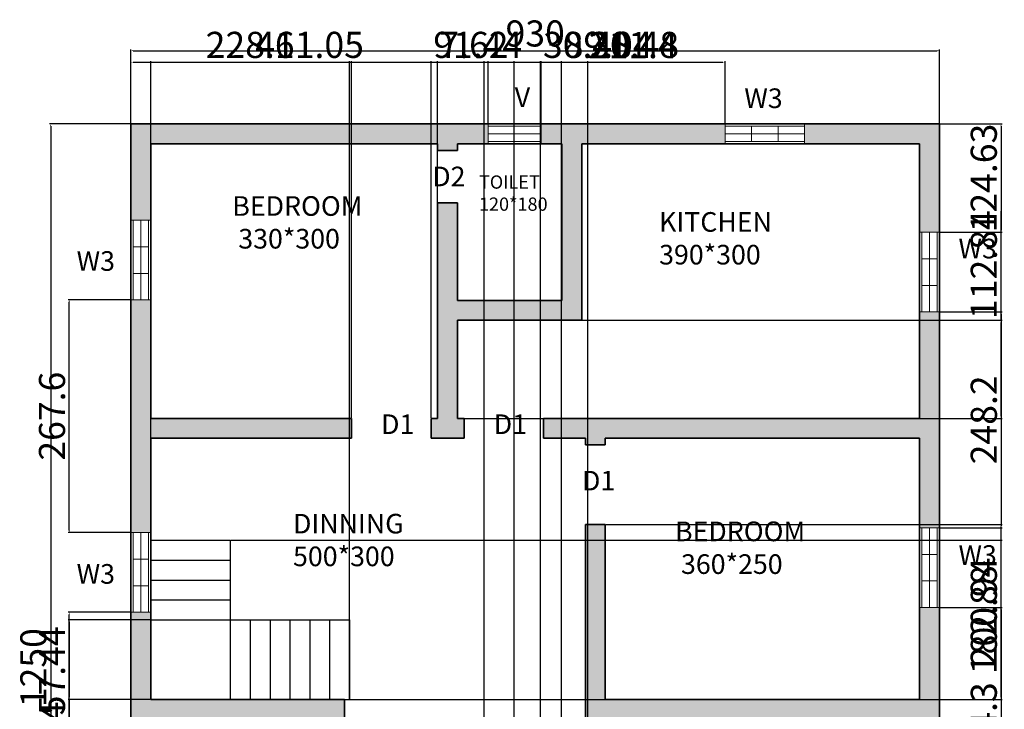
# Model space of a CAD drawing. Units: centimetres. Extents: x 2091 to 3299, y 1401 to 2845.
# Tile 2 of 2: x 2091 to 3224, y 2053 to 2845. Entities that reach past the tile are written whole.
import ezdxf

# ---------------------------------------------------------------- set-up
doc = ezdxf.new("R2010")
doc.units = ezdxf.units.CM
for name, color, linetype, lineweight in [('A-ANNO-DIMS', 2, 'Continuous', 18), ('A-ANNO-TEXT', 7, 'Continuous', 18), ('A-AREA-IDEN', 7, 'Continuous', 25), ('A-FLOR-STRS', 7, 'Continuous', 25), ('A-GLAZ', 4, 'Continuous', 18), ('A-WALL', 7, 'Continuous', 35)]:
    doc.layers.add(name, color=color, linetype=linetype, lineweight=lineweight)
doc.layers.add('A-WALL-PATT', color=18, linetype='Continuous', lineweight=13, true_color=0x000000)
doc.styles.get("Standard").update_dxf_attribs({"font": 'arial.ttf'})
doc.dimstyles.new('ISO-25', dxfattribs={"dimtxt": 30, "dimasz": 2.5, "dimexe": 1.25, "dimexo": 0.625, "dimtad": 1, "dimtxsty": 'Standard', "dimcen": 2.5, "dimadec": 0, "dimazin": 0, "dimtfac": 1, "dimtmove": 0, "dimatfit": 3, "dimfxl": 1, "dimarcsym": 0})

# ---------------------------------------------------------------- blocks, each defined once
blk = doc.blocks.new('*D1')
at = {"layer": 'A-ANNO-DIMS', "color": 0, "lineweight": -2, "transparency": 16777216}
for p, q in [((2218.9, 2726.1), (2218.9, 2810.8)), ((2221.4, 2809.6), (3146.4, 2809.6)), ((3148.9, 2726.1), (3148.9, 2810.8))]:
    blk.add_line(p, q, dxfattribs=at)
at = {"layer": 'A-ANNO-DIMS', "color": 0, "transparency": 16777216}
for points in [[(2221.4, 2810), (2221.4, 2809.1), (2218.9, 2809.6)], [(3146.4, 2810), (3146.4, 2809.1), (3148.9, 2809.6)]]:
    blk.add_solid(points, dxfattribs=at)
at = {"layer": 'Defpoints', "color": 0, "transparency": 16777216}
for p in [(3148.9, 2809.6), (2218.9, 2725.5), (3148.9, 2725.5)]:
    blk.add_point(p, dxfattribs=at)
at = {"layer": 'A-ANNO-DIMS', "color": 0, "transparency": 16777216, "insert": (2683.9, 2825.5), "char_height": 30, "attachment_point": 5}
blk.add_mtext('930', dxfattribs=at)
blk = doc.blocks.new('*D2')
at = {"layer": 'A-ANNO-DIMS', "color": 0, "lineweight": -2, "transparency": 16777216}
for p, q in [((2218.2, 2725.5), (2125.3, 2725.5)), ((2126.6, 2723), (2126.6, 1478)), ((2218.2, 1475.5), (2125.3, 1475.5))]:
    blk.add_line(p, q, dxfattribs=at)
at = {"layer": 'A-ANNO-DIMS', "color": 0, "transparency": 16777216}
for points in [[(2126.2, 2723), (2127, 2723), (2126.6, 2725.5)], [(2126.2, 1478), (2127, 1478), (2126.6, 1475.5)]]:
    blk.add_solid(points, dxfattribs=at)
at = {"layer": 'Defpoints', "color": 0, "transparency": 16777216}
for p in [(2218.9, 2725.5), (2126.6, 1475.5), (2218.9, 1475.5)]:
    blk.add_point(p, dxfattribs=at)
at = {"layer": 'A-ANNO-DIMS', "color": 0, "transparency": 16777216, "insert": (2110.6, 2100.5), "char_height": 30, "attachment_point": 5, "rotation": 90}
blk.add_mtext('1250', dxfattribs=at)
blk = doc.blocks.new('WIN-W3')
for p, q in [((0, 0), (0, 22.9)), ((91.4, 22.9), (91.4, 0)), ((0, 20.3), (91.4, 20.3)), ((0, 11.4), (91.4, 11.4)), ((30.5, 2.5), (30.5, 20.3)), ((61, 2.5), (61, 20.3)), ((91.4, 2.5), (0, 2.5))]:
    blk.add_line(p, q)
blk = doc.blocks.new('VENT-V')
for p, q in [((0, 0), (0, 22.9)), ((61, 22.9), (61, 0)), ((0, 20.3), (61, 20.3)), ((0, 11.4), (61, 11.4)), ((61, 2.5), (0, 2.5))]:
    blk.add_line(p, q)
blk = doc.blocks.new('*D9')
at = {"layer": 'A-ANNO-DIMS', "color": 0, "lineweight": -2, "transparency": 16777216}
for p, q in [((2472.7, 2387.6), (2472.7, 2797.7)), ((2564.1, 2387.6), (2564.1, 2797.7)), ((2475.2, 2796.4), (2561.6, 2796.4)), ((2564.1, 2796.4), (2669, 2796.4))]:
    blk.add_line(p, q, dxfattribs=at)
at = {"layer": 'A-ANNO-DIMS', "color": 0, "transparency": 16777216}
for points in [[(2475.2, 2796.8), (2475.2, 2796), (2472.7, 2796.4)], [(2561.6, 2796.8), (2561.6, 2796), (2564.1, 2796.4)]]:
    blk.add_solid(points, dxfattribs=at)
at = {"layer": 'Defpoints', "color": 0, "transparency": 16777216}
for p in [(2564.1, 2796.4), (2472.7, 2386.9), (2564.1, 2386.9)]:
    blk.add_point(p, dxfattribs=at)
at = {"layer": 'A-ANNO-DIMS', "color": 0, "transparency": 16777216, "insert": (2617.8, 2812.4), "char_height": 30, "attachment_point": 5}
blk.add_mtext('91.44', dxfattribs=at)
blk = doc.blocks.new('*D10')
at = {"layer": 'A-ANNO-DIMS', "color": 0, "lineweight": -2, "transparency": 16777216}
for p, q in [((2564.1, 2387.6), (2564.1, 2797.7)), ((2571.7, 2387.6), (2571.7, 2797.7)), ((2566.6, 2796.4), (2569.2, 2796.4)), ((2571.7, 2796.4), (2652.8, 2796.4))]:
    blk.add_line(p, q, dxfattribs=at)
at = {"layer": 'A-ANNO-DIMS', "color": 0, "transparency": 16777216}
for points in [[(2566.6, 2796.8), (2566.6, 2796), (2564.1, 2796.4)], [(2569.2, 2796.8), (2569.2, 2796), (2571.7, 2796.4)]]:
    blk.add_solid(points, dxfattribs=at)
at = {"layer": 'Defpoints', "color": 0, "transparency": 16777216}
for p in [(2571.7, 2796.4), (2564.1, 2386.9), (2571.7, 2386.9)]:
    blk.add_point(p, dxfattribs=at)
at = {"layer": 'A-ANNO-DIMS', "color": 0, "transparency": 16777216, "insert": (2613.5, 2812.4), "char_height": 30, "attachment_point": 5}
blk.add_mtext('7.62', dxfattribs=at)
blk = doc.blocks.new('*D12')
at = {"layer": 'A-ANNO-DIMS', "color": 0, "lineweight": -2, "transparency": 16777216}
for p, q in [((2625.1, 1721.9), (2625.1, 2797.7)), ((2714.1, 1721.9), (2714.1, 2797.7)), ((2627.6, 2796.4), (2711.6, 2796.4)), ((2714.1, 2796.4), (2819, 2796.4))]:
    blk.add_line(p, q, dxfattribs=at)
at = {"layer": 'A-ANNO-DIMS', "color": 0, "transparency": 16777216}
for points in [[(2627.6, 2796.8), (2627.6, 2796), (2625.1, 2796.4)], [(2711.6, 2796.8), (2711.6, 2796), (2714.1, 2796.4)]]:
    blk.add_solid(points, dxfattribs=at)
at = {"layer": 'Defpoints', "color": 0, "transparency": 16777216}
for p in [(2714.1, 2796.4), (2625.1, 1721.2), (2714.1, 1721.2)]:
    blk.add_point(p, dxfattribs=at)
at = {"layer": 'A-ANNO-DIMS', "color": 0, "transparency": 16777216, "insert": (2767.8, 2812.4), "char_height": 30, "attachment_point": 5}
blk.add_mtext('89.04', dxfattribs=at)
blk = doc.blocks.new('*D13')
at = {"layer": 'A-ANNO-DIMS', "color": 0, "lineweight": -2, "transparency": 16777216}
for p, q in [((2714.1, 1699), (2714.1, 2797.7)), ((2744.6, 1699), (2744.6, 2797.7)), ((2716.6, 2796.4), (2742.1, 2796.4)), ((2744.6, 2796.4), (2849.6, 2796.4))]:
    blk.add_line(p, q, dxfattribs=at)
at = {"layer": 'A-ANNO-DIMS', "color": 0, "transparency": 16777216}
for points in [[(2716.6, 2796.8), (2716.6, 2796), (2714.1, 2796.4)], [(2742.1, 2796.8), (2742.1, 2796), (2744.6, 2796.4)]]:
    blk.add_solid(points, dxfattribs=at)
at = {"layer": 'Defpoints', "color": 0, "transparency": 16777216}
for p in [(2744.6, 2796.4), (2714.1, 1698.4), (2744.6, 1698.4)]:
    blk.add_point(p, dxfattribs=at)
at = {"layer": 'A-ANNO-DIMS', "color": 0, "transparency": 16777216, "insert": (2798.3, 2812.4), "char_height": 30, "attachment_point": 5}
blk.add_mtext('30.48', dxfattribs=at)
blk = doc.blocks.new('*D19')
at = {"layer": 'A-ANNO-DIMS', "color": 0, "lineweight": -2, "transparency": 16777216}
for p, q in [((2333.8, 2247), (3221, 2247)), ((3219.8, 2066.6), (3219.8, 2244.5)), ((2333.8, 2064.1), (3221, 2064.1))]:
    blk.add_line(p, q, dxfattribs=at)
at = {"layer": 'A-ANNO-DIMS', "color": 0, "transparency": 16777216}
for points in [[(3219.3, 2244.5), (3220.2, 2244.5), (3219.8, 2247)], [(3219.3, 2066.6), (3220.2, 2066.6), (3219.8, 2064.1)]]:
    blk.add_solid(points, dxfattribs=at)
at = {"layer": 'Defpoints', "color": 0, "transparency": 16777216}
for p in [(2333.2, 2247), (3219.8, 2247), (2333.2, 2064.1)]:
    blk.add_point(p, dxfattribs=at)
at = {"layer": 'A-ANNO-DIMS', "color": 0, "transparency": 16777216, "insert": (3203.8, 2155.5), "char_height": 30, "attachment_point": 5, "rotation": 90}
blk.add_mtext('182.88', dxfattribs=at)
blk = doc.blocks.new('*D20')
at = {"layer": 'A-ANNO-DIMS', "color": 0, "lineweight": -2, "transparency": 16777216}
for p, q in [((2241.7, 2064.7), (2241.7, 2797.7)), ((2470.3, 2064.7), (2470.3, 2797.7)), ((2244.2, 2796.4), (2467.8, 2796.4))]:
    blk.add_line(p, q, dxfattribs=at)
at = {"layer": 'A-ANNO-DIMS', "color": 0, "transparency": 16777216}
for points in [[(2244.2, 2796.8), (2244.2, 2796), (2241.7, 2796.4)], [(2467.8, 2796.8), (2467.8, 2796), (2470.3, 2796.4)]]:
    blk.add_solid(points, dxfattribs=at)
at = {"layer": 'Defpoints', "color": 0, "transparency": 16777216}
for p in [(2470.3, 2796.4), (2241.7, 2064.1), (2470.3, 2064.1)]:
    blk.add_point(p, dxfattribs=at)
at = {"layer": 'A-ANNO-DIMS', "color": 0, "transparency": 16777216, "insert": (2356, 2812.4), "char_height": 30, "attachment_point": 5}
blk.add_mtext('228.6', dxfattribs=at)
blk = doc.blocks.new('*D21')
at = {"layer": 'A-ANNO-DIMS', "color": 0, "lineweight": -2, "transparency": 16777216}
for p, q in [((2241.1, 2155.5), (2146.7, 2155.5)), ((2148, 2153), (2148, 2066.6)), ((2241.1, 2064.1), (2146.7, 2064.1)), ((2148, 2064.1), (2148, 1959.2))]:
    blk.add_line(p, q, dxfattribs=at)
at = {"layer": 'A-ANNO-DIMS', "color": 0, "transparency": 16777216}
for points in [[(2147.5, 2153), (2148.4, 2153), (2148, 2155.5)], [(2147.5, 2066.6), (2148.4, 2066.6), (2148, 2064.1)]]:
    blk.add_solid(points, dxfattribs=at)
at = {"layer": 'Defpoints', "color": 0, "transparency": 16777216}
for p in [(2241.7, 2155.5), (2148, 2064.1), (2241.7, 2064.1)]:
    blk.add_point(p, dxfattribs=at)
at = {"layer": 'A-ANNO-DIMS', "color": 0, "transparency": 16777216, "insert": (2132, 2010.4), "char_height": 30, "attachment_point": 5, "rotation": 90}
blk.add_mtext('91.44', dxfattribs=at)
blk = doc.blocks.new('*D24')
at = {"layer": 'A-ANNO-DIMS', "color": 0, "lineweight": -2, "transparency": 16777216}
for p, q in [((2659.7, 1499), (2659.7, 2797.7)), ((2690.2, 1499), (2690.2, 2797.7)), ((2662.2, 2796.4), (2687.7, 2796.4)), ((2690.2, 2796.4), (2795.2, 2796.4))]:
    blk.add_line(p, q, dxfattribs=at)
at = {"layer": 'A-ANNO-DIMS', "color": 0, "transparency": 16777216}
for points in [[(2662.2, 2796.8), (2662.2, 2796), (2659.7, 2796.4)], [(2687.7, 2796.8), (2687.7, 2796), (2690.2, 2796.4)]]:
    blk.add_solid(points, dxfattribs=at)
at = {"layer": 'Defpoints', "color": 0, "transparency": 16777216}
for p in [(2690.2, 2796.4), (2659.7, 1498.4), (2690.2, 1498.4)]:
    blk.add_point(p, dxfattribs=at)
at = {"layer": 'A-ANNO-DIMS', "color": 0, "transparency": 16777216, "insert": (2744, 2812.4), "char_height": 30, "attachment_point": 5}
blk.add_mtext('30.48', dxfattribs=at)
blk = doc.blocks.new('*D27')
at = {"layer": 'A-ANNO-DIMS', "color": 0, "lineweight": -2, "transparency": 16777216}
for p, q in [((2218.2, 2164.2), (2146.7, 2164.2)), ((2148, 2009.3), (2148, 2161.7)), ((2218.2, 2006.8), (2146.7, 2006.8))]:
    blk.add_line(p, q, dxfattribs=at)
at = {"layer": 'A-ANNO-DIMS', "color": 0, "transparency": 16777216}
for points in [[(2147.5, 2161.7), (2148.4, 2161.7), (2148, 2164.2)], [(2147.5, 2009.3), (2148.4, 2009.3), (2148, 2006.8)]]:
    blk.add_solid(points, dxfattribs=at)
at = {"layer": 'Defpoints', "color": 0, "transparency": 16777216}
for p in [(2148, 2164.2), (2218.9, 2164.2), (2218.9, 2006.8)]:
    blk.add_point(p, dxfattribs=at)
at = {"layer": 'A-ANNO-DIMS', "color": 0, "transparency": 16777216, "insert": (2132, 2085.5), "char_height": 30, "attachment_point": 5, "rotation": 90}
blk.add_mtext('157.44', dxfattribs=at)
blk = doc.blocks.new('*D28')
at = {"layer": 'A-ANNO-DIMS', "color": 0, "lineweight": -2, "transparency": 16777216}
for p, q in [((2218.2, 2523.3), (2146.7, 2523.3)), ((2148, 2258.2), (2148, 2520.8)), ((2218.2, 2255.7), (2146.7, 2255.7))]:
    blk.add_line(p, q, dxfattribs=at)
at = {"layer": 'A-ANNO-DIMS', "color": 0, "transparency": 16777216}
for points in [[(2147.5, 2520.8), (2148.4, 2520.8), (2148, 2523.3)], [(2147.5, 2258.2), (2148.4, 2258.2), (2148, 2255.7)]]:
    blk.add_solid(points, dxfattribs=at)
at = {"layer": 'Defpoints', "color": 0, "transparency": 16777216}
for p in [(2148, 2523.3), (2218.9, 2523.3), (2218.9, 2255.7)]:
    blk.add_point(p, dxfattribs=at)
at = {"layer": 'A-ANNO-DIMS', "color": 0, "transparency": 16777216, "insert": (2132, 2389.5), "char_height": 30, "attachment_point": 5, "rotation": 90}
blk.add_mtext('267.6', dxfattribs=at)
blk = doc.blocks.new('*D29')
at = {"layer": 'A-ANNO-DIMS', "color": 0, "lineweight": -2, "transparency": 16777216}
for p, q in [((2218.9, 2726.1), (2218.9, 2797.7)), ((2629.9, 2726.1), (2629.9, 2797.7)), ((2221.4, 2796.4), (2627.4, 2796.4))]:
    blk.add_line(p, q, dxfattribs=at)
at = {"layer": 'A-ANNO-DIMS', "color": 0, "transparency": 16777216}
for points in [[(2221.4, 2796.8), (2221.4, 2796), (2218.9, 2796.4)], [(2627.4, 2796.8), (2627.4, 2796), (2629.9, 2796.4)]]:
    blk.add_solid(points, dxfattribs=at)
at = {"layer": 'Defpoints', "color": 0, "transparency": 16777216}
for p in [(2629.9, 2796.4), (2218.9, 2725.5), (2629.9, 2725.5)]:
    blk.add_point(p, dxfattribs=at)
at = {"layer": 'A-ANNO-DIMS', "color": 0, "transparency": 16777216, "insert": (2424.4, 2812.4), "char_height": 30, "attachment_point": 5}
blk.add_mtext('411.05', dxfattribs=at)
blk = doc.blocks.new('*D30')
at = {"layer": 'A-ANNO-DIMS', "color": 0, "lineweight": -2, "transparency": 16777216}
for p, q in [((2690.9, 2726.1), (2690.9, 2797.7)), ((2902.3, 2726.1), (2902.3, 2797.7)), ((2693.4, 2796.4), (2899.8, 2796.4))]:
    blk.add_line(p, q, dxfattribs=at)
at = {"layer": 'A-ANNO-DIMS', "color": 0, "transparency": 16777216}
for points in [[(2693.4, 2796.8), (2693.4, 2796), (2690.9, 2796.4)], [(2899.8, 2796.8), (2899.8, 2796), (2902.3, 2796.4)]]:
    blk.add_solid(points, dxfattribs=at)
at = {"layer": 'Defpoints', "color": 0, "transparency": 16777216}
for p in [(2902.3, 2796.4), (2690.9, 2725.5), (2902.3, 2725.5)]:
    blk.add_point(p, dxfattribs=at)
at = {"layer": 'A-ANNO-DIMS', "color": 0, "transparency": 16777216, "insert": (2796.6, 2812.1), "char_height": 30, "attachment_point": 5}
blk.add_mtext('211.4', dxfattribs=at)
blk = doc.blocks.new('*D31')
at = {"layer": 'A-ANNO-DIMS', "color": 0, "lineweight": -2, "transparency": 16777216}
for p, q in [((3149.5, 2725.5), (3221, 2725.5)), ((3219.8, 2723), (3219.8, 2603.4)), ((3149.5, 2600.9), (3221, 2600.9))]:
    blk.add_line(p, q, dxfattribs=at)
at = {"layer": 'A-ANNO-DIMS', "color": 0, "transparency": 16777216}
for points in [[(3219.3, 2723), (3220.2, 2723), (3219.8, 2725.5)], [(3219.3, 2603.4), (3220.2, 2603.4), (3219.8, 2600.9)]]:
    blk.add_solid(points, dxfattribs=at)
at = {"layer": 'Defpoints', "color": 0, "transparency": 16777216}
for p in [(3148.9, 2725.5), (3148.9, 2600.9), (3219.8, 2600.9)]:
    blk.add_point(p, dxfattribs=at)
at = {"layer": 'A-ANNO-DIMS', "color": 0, "transparency": 16777216, "insert": (3203.8, 2663.2), "char_height": 30, "attachment_point": 5, "rotation": 90}
blk.add_mtext('124.63', dxfattribs=at)
blk = doc.blocks.new('*D32')
at = {"layer": 'A-ANNO-DIMS', "color": 0, "lineweight": -2, "transparency": 16777216}
for p, q in [((3149.5, 2509.4), (3221, 2509.4)), ((3219.8, 2506.9), (3219.8, 2263.7)), ((3149.5, 2261.2), (3221, 2261.2))]:
    blk.add_line(p, q, dxfattribs=at)
at = {"layer": 'A-ANNO-DIMS', "color": 0, "transparency": 16777216}
for points in [[(3219.3, 2506.9), (3220.2, 2506.9), (3219.8, 2509.4)], [(3219.3, 2263.7), (3220.2, 2263.7), (3219.8, 2261.2)]]:
    blk.add_solid(points, dxfattribs=at)
at = {"layer": 'Defpoints', "color": 0, "transparency": 16777216}
for p in [(3148.9, 2509.4), (3148.9, 2261.2), (3219.8, 2261.2)]:
    blk.add_point(p, dxfattribs=at)
at = {"layer": 'A-ANNO-DIMS', "color": 0, "transparency": 16777216, "insert": (3203.8, 2385.3), "char_height": 30, "attachment_point": 5, "rotation": 90}
blk.add_mtext('248.2', dxfattribs=at)
blk = doc.blocks.new('*D33')
at = {"layer": 'A-ANNO-DIMS', "color": 0, "lineweight": -2, "transparency": 16777216}
for p, q in [((3149.5, 2169.8), (3221, 2169.8)), ((3219.8, 2167.3), (3219.8, 1898)), ((3149.5, 1895.5), (3221, 1895.5))]:
    blk.add_line(p, q, dxfattribs=at)
at = {"layer": 'A-ANNO-DIMS', "color": 0, "transparency": 16777216}
for points in [[(3219.3, 2167.3), (3220.2, 2167.3), (3219.8, 2169.8)], [(3219.3, 1898), (3220.2, 1898), (3219.8, 1895.5)]]:
    blk.add_solid(points, dxfattribs=at)
at = {"layer": 'Defpoints', "color": 0, "transparency": 16777216}
for p in [(3148.9, 2169.8), (3148.9, 1895.5), (3219.8, 1895.5)]:
    blk.add_point(p, dxfattribs=at)
at = {"layer": 'A-ANNO-DIMS', "color": 0, "transparency": 16777216, "insert": (3203.8, 2032.6), "char_height": 30, "attachment_point": 5, "rotation": 90}
blk.add_mtext('274.3', dxfattribs=at)
blk = doc.blocks.new('*D37')
at = {"layer": 'A-ANNO-DIMS', "color": 0, "lineweight": -2, "transparency": 16777216}
for p, q in [((2765.2, 2265), (3221, 2265)), ((3219.8, 2066.6), (3219.8, 2262.5)), ((2765.2, 2064.1), (3221, 2064.1))]:
    blk.add_line(p, q, dxfattribs=at)
at = {"layer": 'A-ANNO-DIMS', "color": 0, "transparency": 16777216}
for points in [[(3219.3, 2262.5), (3220.2, 2262.5), (3219.8, 2265)], [(3219.3, 2066.6), (3220.2, 2066.6), (3219.8, 2064.1)]]:
    blk.add_solid(points, dxfattribs=at)
at = {"layer": 'Defpoints', "color": 0, "transparency": 16777216}
for p in [(2764.6, 2265), (3219.8, 2265), (2764.6, 2064.1)]:
    blk.add_point(p, dxfattribs=at)
at = {"layer": 'A-ANNO-DIMS', "color": 0, "transparency": 16777216, "insert": (3203.8, 2164.6), "char_height": 30, "attachment_point": 5, "rotation": 90}
blk.add_mtext('200.94', dxfattribs=at)
blk = doc.blocks.new('*D38')
at = {"layer": 'A-ANNO-DIMS', "color": 0, "lineweight": -2, "transparency": 16777216}
for p, q in [((3219.8, 2499.8), (3219.8, 2625.1)), ((2595.2, 2499.8), (3221, 2499.8)), ((3219.8, 2389.4), (3219.8, 2497.3)), ((2595.2, 2386.9), (3221, 2386.9))]:
    blk.add_line(p, q, dxfattribs=at)
at = {"layer": 'A-ANNO-DIMS', "color": 0, "transparency": 16777216}
for points in [[(3219.3, 2497.3), (3220.2, 2497.3), (3219.8, 2499.8)], [(3219.3, 2389.4), (3220.2, 2389.4), (3219.8, 2386.9)]]:
    blk.add_solid(points, dxfattribs=at)
at = {"layer": 'Defpoints', "color": 0, "transparency": 16777216}
for p in [(2594.6, 2499.8), (3219.8, 2499.8), (2594.6, 2386.9)]:
    blk.add_point(p, dxfattribs=at)
at = {"layer": 'A-ANNO-DIMS', "color": 0, "transparency": 16777216, "insert": (3203.8, 2563.7), "char_height": 30, "attachment_point": 5, "rotation": 90}
blk.add_mtext('112.84', dxfattribs=at)

msp = doc.modelspace()

# ---------------------------------------------------------------- hatches: boundary and pattern name
at = {"layer": 'A-WALL-PATT'}
h = msp.add_hatch(color=256, dxfattribs=at)
h.dxf.hatch_style = 1
h.paths.add_polyline_path([(2629.919, 2725.51), (2218.865, 2725.51), (2218.865, 2614.708), (2241.725, 2614.708), (2241.725, 2702.65), (2571.725, 2702.65), (2571.725, 2695.03), (2594.585, 2695.03), (2594.585, 2702.65), (2629.919, 2702.65)])
h.paths.add_polyline_path([(2902.29, 2725.51), (2690.879, 2725.51), (2690.879, 2702.65), (2714.585, 2702.65), (2714.585, 2522.65), (2594.585, 2522.65), (2594.585, 2634.77), (2571.725, 2634.77), (2571.725, 2386.95), (2564.105, 2386.95), (2564.105, 2364.09), (2602.205, 2364.09), (2602.205, 2386.95), (2594.585, 2386.95), (2594.585, 2499.79), (2737.445, 2499.79), (2737.445, 2702.65), (2902.29, 2702.65)])
h.paths.add_polyline_path([(3148.865, 2725.51), (2993.73, 2725.51), (2993.73, 2702.65), (3126.005, 2702.65), (3126.005, 2600.88), (3148.865, 2600.88)])
h.paths.add_polyline_path([(3148.865, 2509.44), (3126.005, 2509.44), (3126.005, 2386.95), (2693.645, 2386.95), (2693.645, 2364.09), (2741.725, 2364.09), (2741.725, 2356.47), (2764.585, 2356.47), (2764.585, 2364.09), (3126.005, 2364.09), (3126.005, 2261.228), (3148.865, 2261.228)])
h.paths.add_polyline_path([(2472.665, 2386.95), (2241.725, 2386.95), (2241.725, 2523.268), (2218.865, 2523.268), (2218.865, 2255.666), (2241.725, 2255.666), (2241.725, 2364.09), (2472.665, 2364.09)])
h.paths.add_polyline_path([(3148.865, 2169.788), (3126.005, 2169.788), (3126.005, 2064.09), (2764.585, 2064.09), (2764.585, 2265.03), (2741.725, 2265.03), (2741.725, 1921.23), (2764.585, 1921.23), (2764.585, 2041.23), (3126.005, 2041.23), (3126.005, 1895.472), (3148.865, 1895.472)])
h.paths.add_polyline_path([(3148.865, 1804.032), (3126.005, 1804.032), (3126.005, 1671.23), (3095.525, 1671.23), (3095.525, 1648.37), (3148.865, 1648.37)])
h.paths.add_polyline_path([(2241.725, 2155.53), (2241.725, 2164.226), (2218.865, 2164.226), (2218.865, 2006.784), (2241.725, 2006.784), (2241.725, 2041.23), (2441.725, 2041.23), (2441.725, 1921.23), (2434.105, 1921.23), (2434.105, 1898.37), (2472.665, 1898.37), (2472.665, 1921.23), (2464.585, 1921.23), (2464.585, 2064.09), (2241.725, 2064.09)])
h.paths.add_polyline_path([(2241.725, 1898.37), (2373.145, 1898.37), (2373.145, 1921.23), (2241.725, 1921.23), (2241.725, 1945.824), (2218.865, 1945.824), (2218.865, 1747.285), (2241.725, 1747.285)])
h.paths.add_polyline_path([(2241.725, 1655.845), (2218.865, 1655.845), (2218.865, 1475.51), (2363.981, 1475.51), (2363.981, 1498.37), (2241.725, 1498.37)])
h.paths.add_polyline_path([(2594.585, 1921.23), (2564.105, 1921.23), (2564.105, 1898.37), (2571.725, 1898.37), (2571.725, 1498.37), (2455.421, 1498.37), (2455.421, 1475.51), (2659.718, 1475.51), (2659.718, 1498.37), (2594.585, 1498.37), (2594.585, 1698.37), (2625.065, 1698.37), (2625.065, 1721.23), (2594.585, 1721.23)])
h.paths.add_polyline_path([(2767.445, 1721.23), (2767.445, 1751.71), (2744.585, 1751.71), (2744.585, 1721.23), (2714.105, 1721.23), (2714.105, 1698.37), (2744.585, 1698.37), (2744.585, 1498.37), (2690.198, 1498.37), (2690.198, 1475.51), (2767.445, 1475.51)])
h.paths.add_polyline_path([(3148.865, 1536.968), (3126.005, 1536.968), (3126.005, 1514.108), (3148.865, 1514.108)])
h.paths.add_polyline_path([(2919.845, 1671.23), (2889.365, 1671.23), (2889.365, 1648.37), (2919.845, 1648.37)])

# ---------------------------------------------------------------- linework, layer by layer
at = {"layer": 'A-FLOR-STRS'}
for p, q in [((2241.725, 2246.97), (2333.165, 2246.97)), ((2333.165, 2246.97), (2333.165, 2155.53)), ((2241.725, 2224.11), (2333.165, 2224.11)), ((2241.725, 2201.25), (2333.165, 2201.25)), ((2241.725, 2178.39), (2333.165, 2178.39)), ((2241.725, 2064.09), (2241.725, 2155.53)), ((2241.725, 2155.53), (2333.165, 2155.53)), ((2333.165, 2155.53), (2333.165, 2064.09)), ((2333.165, 2155.53), (2470.325, 2155.53)), ((2356.025, 2155.53), (2356.025, 2064.09)), ((2378.885, 2155.53), (2378.885, 2064.09)), ((2401.745, 2155.53), (2401.745, 2064.09)), ((2424.605, 2155.53), (2424.605, 2064.09)), ((2447.465, 2155.53), (2447.465, 2064.09)), ((2470.325, 2155.53), (2470.325, 2064.09)), ((2241.725, 2147.203), (2241.725, 2147.203))]:
    msp.add_line(p, q, dxfattribs=at)
at = {"layer": 'A-WALL'}
for p, q in [((2218.865, 2725.51), (3148.865, 2725.51)), ((2218.865, 1475.51), (2218.865, 2725.51)), ((3148.865, 2725.51), (3148.865, 1483.628)), ((2241.725, 2702.65), (2571.725, 2702.65)), ((2241.725, 2386.95), (2241.725, 2702.65)), ((2571.725, 2695.03), (2571.725, 2702.65)), ((2594.585, 2695.03), (2594.585, 2702.65)), ((2594.585, 2702.65), (2714.585, 2702.65)), ((2594.585, 2702.65), (2714.585, 2702.65)), ((2714.585, 2522.65), (2714.585, 2702.65)), ((2737.445, 2499.79), (2737.445, 2702.65)), ((2737.445, 2702.65), (3126.005, 2702.65)), ((3126.005, 2702.65), (3126.005, 2386.95)), ((2594.585, 2695.03), (2571.725, 2695.03)), ((2571.725, 2386.95), (2571.725, 2634.77)), ((2594.585, 2634.77), (2571.725, 2634.77)), ((2594.585, 2522.65), (2594.585, 2634.77)), ((2594.585, 2522.65), (2714.585, 2522.65)), ((2594.585, 2386.95), (2594.585, 2499.79)), ((2594.585, 2499.79), (2737.445, 2499.79)), ((2472.665, 2386.95), (2241.725, 2386.95)), ((2472.665, 2364.09), (2472.665, 2386.95)), ((2564.105, 2364.09), (2564.105, 2386.95)), ((2571.725, 2386.95), (2564.105, 2386.95)), ((2594.585, 2386.95), (2602.205, 2386.95)), ((2602.205, 2386.95), (2594.585, 2386.95)), ((2602.205, 2386.95), (2602.205, 2364.09)), ((3126.005, 2386.95), (2693.645, 2386.95)), ((2693.645, 2386.95), (2693.645, 2364.09)), ((2472.665, 2364.09), (2241.725, 2364.09)), ((2241.725, 2064.09), (2241.725, 2364.09)), ((2602.205, 2364.09), (2564.105, 2364.09)), ((2741.725, 2364.09), (2693.645, 2364.09)), ((2741.725, 2364.09), (2741.725, 2356.47)), ((2764.585, 2356.47), (2741.725, 2356.47)), ((3126.005, 2364.09), (2764.585, 2364.09)), ((2764.585, 2364.09), (2764.585, 2356.47)), ((3126.005, 2364.09), (3126.005, 2064.09)), ((2764.585, 2265.03), (2741.725, 2265.03)), ((2741.725, 2265.03), (2741.725, 2064.09)), ((2741.725, 1921.23), (2741.725, 2265.03)), ((2764.585, 2265.03), (2764.585, 2064.09)), ((2464.585, 2064.09), (2241.725, 2064.09)), ((2464.585, 2064.09), (2464.585, 1921.23)), ((3126.005, 2064.09), (2764.585, 2064.09))]:
    msp.add_line(p, q, dxfattribs=at)

# ---------------------------------------------------------------- block references
at = {"layer": 'A-GLAZ'}
for name, p in [('VENT-V', (2629.919, 2702.65)), ('WIN-W3', (2902.29, 2702.65))]:
    msp.add_blockref(name, p, dxfattribs=at)
for p, rotation in [((2218.866, 2614.707), 270.0000000000007), ((3126.006, 2600.879), 270.0000000000001), ((2218.866, 2255.665), 270.0000000000002), ((3126.006, 2261.227), 270.0000000000001)]:
    msp.add_blockref('WIN-W3', p, dxfattribs=dict(at, rotation=rotation))

# ---------------------------------------------------------------- texts
at = {"layer": 'A-ANNO-TEXT', "char_height": 22.56, "attachment_point": 1}
for s, width, insert in [('V', 39.89904, (2660.399, 2767.394)), ('W3', 162.65151, (2924.469, 2766.231)), ('D2', 22.59147, (2565.478, 2676.309)), ('W3', 162.65151, (3170.799, 2593.452)), ('W3', 162.65151, (2156.466, 2579.16)), ('D1', 21.81012, (2506.661, 2391.583)), ('D1', 21.81012, (2636.239, 2391.583)), ('D1', 21.81012, (2737.744, 2326.703)), ('W3', 162.65151, (3170.799, 2241.231)), ('W3', 162.65151, (2156.466, 2219.517))]:
    msp.add_mtext_dynamic_manual_height_columns(s, width=width, gutter_width=12.5, heights=[0], dxfattribs=dict(at, insert=insert))
at = {"layer": 'A-AREA-IDEN', "attachment_point": 1}
for s, width, insert, char_height in [('TOILET \\P120*180', 61.36767, (2619.251, 2666.251), 15.24), ('BEDROOM \\P 330*300', 153.02066, (2335.525, 2642.361), 22.56), ('KITCHEN\\P390*300', 150.62972, (2826.467, 2624.045), 22.56), ('DINNING\\P500*300', 206.52607, (2405.386, 2277.3), 22.56), ('BEDROOM \\P 360*250', 153.02066, (2844.754, 2268.409), 22.56)]:
    msp.add_mtext_dynamic_manual_height_columns(s, width=width, gutter_width=12.5, heights=[0], dxfattribs=dict(at, insert=insert, char_height=char_height))

# ---------------------------------------------------------------- dimensions: what is measured, and where the dimension line sits
at = {"layer": 'A-ANNO-DIMS'}
for base, p1, p2, override, picture, middle in [((3148.865, 2809.563), (2218.865, 2725.51), (3148.865, 2725.51), {"dimclrd": 0, "dimclre": 0, "dimclrt": 0}, '*D1', (2683.865, 2825.515)), ((2629.919, 2796.41), (2218.865, 2725.51), (2629.919, 2725.51), {"dimdec": 2, "dimlfac": 1, "dimrnd": 0, "dimzin": 0, "dimdsep": 46, "dimlunit": 2}, '*D29', (2424.392, 2812.352)), ((2470.325, 2796.41), (2241.725, 2064.09), (2470.325, 2064.09), {"dimdec": 1, "dimlfac": 1, "dimrnd": 0, "dimzin": 0, "dimdsep": 46, "dimlunit": 2}, '*D20', (2356.025, 2812.352)), ((2564.105, 2796.41), (2472.665, 2386.95), (2564.105, 2386.95), {"dimdec": 2, "dimlfac": 1, "dimrnd": 0, "dimzin": 0, "dimdsep": 46, "dimlunit": 2}, '*D9', (2617.786, 2812.352)), ((2571.725, 2796.41), (2564.105, 2386.95), (2571.725, 2386.95), {"dimdec": 2, "dimlfac": 1, "dimrnd": 0, "dimzin": 0, "dimdsep": 46, "dimlunit": 2}, '*D10', (2613.537, 2812.352)), ((2714.105, 2796.41), (2625.065, 1721.23), (2714.105, 1721.23), {"dimdec": 2, "dimlfac": 1, "dimrnd": 0, "dimzin": 0, "dimdsep": 46, "dimlunit": 2}, '*D12', (2767.807, 2812.352)), ((2690.198, 2796.41), (2659.718, 1498.37), (2690.198, 1498.37), {"dimdec": 2, "dimlfac": 1, "dimrnd": 0, "dimzin": 0, "dimdsep": 46, "dimlunit": 2}, '*D24', (2743.961, 2812.362)), ((2902.29, 2796.41), (2690.879, 2725.51), (2902.29, 2725.51), {"dimdec": 1, "dimlfac": 1, "dimrnd": 0, "dimzin": 0, "dimdsep": 46, "dimlunit": 2}, '*D30', (2796.585, 2812.096)), ((2744.585, 2796.41), (2714.105, 1698.37), (2744.585, 1698.37), {"dimdec": 2, "dimlfac": 1, "dimrnd": 0, "dimzin": 0, "dimdsep": 46, "dimlunit": 2}, '*D13', (2798.348, 2812.362))]:
    dim = msp.add_linear_dim(base=base, p1=p1, p2=p2, dimstyle='ISO-25', override=override, dxfattribs=at)
    dim.commit()
    dim.dimension.update_dxf_attribs({"geometry": picture, "text_midpoint": middle})
for base, p1, p2, override, picture, middle in [((2126.587, 1475.51), (2218.865, 2725.51), (2218.865, 1475.51), {"dimclrd": 0, "dimclre": 0, "dimclrt": 0}, '*D2', (2110.644, 2100.51)), ((3219.765, 2600.88), (3148.865, 2725.51), (3148.865, 2600.88), {"dimdec": 2, "dimlfac": 1, "dimrnd": 0, "dimzin": 0, "dimdsep": 46, "dimlunit": 2}, '*D31', (3203.813, 2663.195)), ((3219.765, 2499.79), (2594.585, 2386.95), (2594.585, 2499.79), {"dimdec": 2, "dimlfac": 1, "dimrnd": 0, "dimzin": 0, "dimdsep": 46, "dimlunit": 2}, '*D38', (3203.823, 2563.713)), ((2147.965, 2523.268), (2218.865, 2255.666), (2218.865, 2523.268), {"dimdec": 1, "dimlfac": 1, "dimrnd": 0, "dimzin": 0, "dimdsep": 46, "dimlunit": 2}, '*D28', (2132.023, 2389.467)), ((3219.765, 2261.228), (3148.865, 2509.44), (3148.865, 2261.228), {"dimdec": 1, "dimlfac": 1, "dimrnd": 0, "dimzin": 0, "dimdsep": 46, "dimlunit": 2}, '*D32', (3203.823, 2385.334)), ((3219.765, 2265.03), (2764.585, 2064.09), (2764.585, 2265.03), {"dimdec": 2, "dimlfac": 1, "dimrnd": 0, "dimzin": 0, "dimdsep": 46, "dimlunit": 2}, '*D37', (3203.823, 2164.56)), ((3219.765, 2246.97), (2333.165, 2064.09), (2333.165, 2246.97), {"dimdec": 2, "dimlfac": 1, "dimrnd": 0, "dimzin": 0, "dimdsep": 46, "dimlunit": 2}, '*D19', (3203.823, 2155.53)), ((2147.965, 2164.226), (2218.865, 2006.784), (2218.865, 2164.226), {"dimdec": 2, "dimlfac": 1, "dimrnd": 0, "dimzin": 0, "dimdsep": 46, "dimlunit": 2}, '*D27', (2132.023, 2085.505)), ((3219.765, 1895.472), (3148.865, 2169.788), (3148.865, 1895.472), {"dimdec": 1, "dimlfac": 1, "dimrnd": 0, "dimzin": 0, "dimdsep": 46, "dimlunit": 2}, '*D33', (3203.813, 2032.63)), ((2147.965, 2064.09), (2241.725, 2155.53), (2241.725, 2064.09), {"dimdec": 2, "dimlfac": 1, "dimrnd": 0, "dimzin": 0, "dimdsep": 46, "dimlunit": 2}, '*D21', (2132.023, 2010.409))]:
    dim = msp.add_linear_dim(base=base, p1=p1, p2=p2, angle=90, dimstyle='ISO-25', override=override, dxfattribs=at)
    dim.commit()
    dim.dimension.update_dxf_attribs({"geometry": picture, "text_midpoint": middle})

doc.saveas('drawing.dxf')
